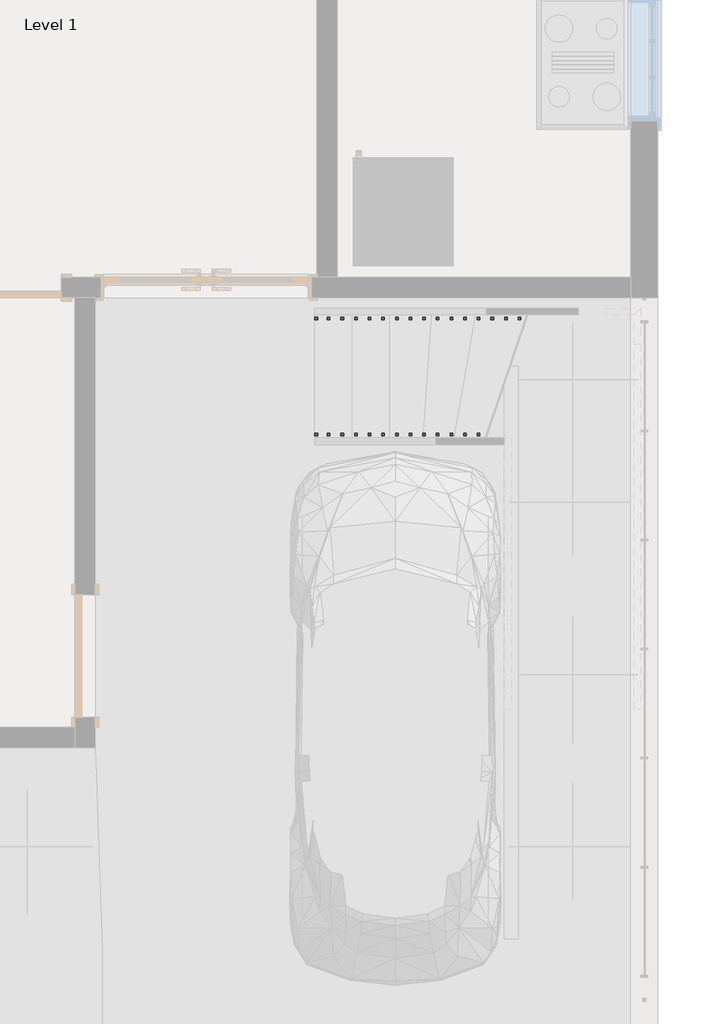
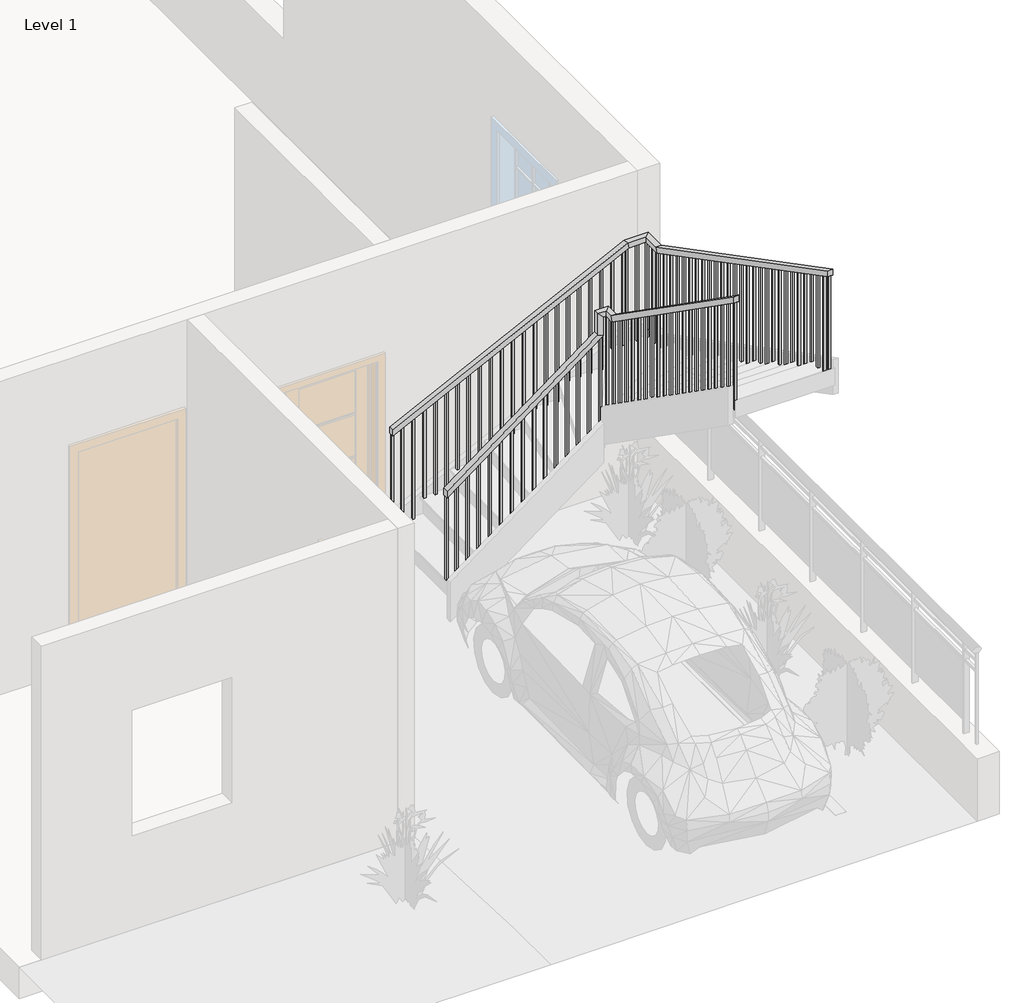
# One storey, part 2 of 3: 2 railings.
"""IFC4 building model written with IfcOpenShell, lengths in millimetres."""

from ifc_helpers import new_model, si_unit, frame, origin, place, context, project, spatial, polyline, outline, extrude, faceted_brep, element, save

model = new_model("IFC4")

# Units and contexts
model_context = context("Model", 3, world=origin())
ifc_project = project(units=[si_unit("LENGTHUNIT", "METRE", prefix="MILLI")], contexts=[model_context])

# Site, building, storey
site = spatial("IfcSite", under=ifc_project)
building = spatial("IfcBuilding", under=site)
storey = spatial("IfcBuildingStorey", under=building, Name="Level 1", Elevation=0.0)

# Railings
placement = place(None, origin())
element("IfcRailing", 1, ObjectType="Handrail - Rectangular", at=placement, inside=storey, context=model_context, shape_type="SolidModel", body=[
    faceted_brep([(2176.6969821, -750.949605, 1382.8377299), (2176.6969821, -750.949605, 1319.4090472), (2176.6969821, -801.749605, 1319.4090472), (2176.6969821, -801.749605, 1382.8377299), (3563.2339716, -750.949605, 2419.4929952), (3614.0339716, -750.949605, 2394.0453313), (3614.0339716, -801.749605, 2394.0453313), (3563.2339716, -801.749605, 2419.4929952), (3563.2339716, -750.949605, 2625.457216), (3614.0339716, -750.949605, 2574.657216), (3614.0339716, -801.749605, 2574.657216), (3563.2339716, -801.749605, 2625.457216), (3690.2339716, -750.949605, 2625.457216), (3690.2339716, -750.949605, 2574.657216), (3639.4339716, -801.749605, 2574.657216), (3639.4339716, -801.749605, 2625.457216), (3690.2339716, -877.949605, 2625.457216), (3690.2339716, -893.9792408, 2574.657216), (3639.4339716, -893.9792408, 2574.657216), (3639.4339716, -877.949605, 2625.457216), (3690.2339716, -2823.2865945, 3988.8904479), (3639.4339716, -2823.2865945, 3988.8904479), (3639.4339716, -2823.2865945, 3926.8557166), (3690.2339716, -2823.2865945, 3926.8557166)], [[[0, 1, 2, 3]], [[1, 0, 4, 5]], [[2, 1, 5, 6]], [[3, 2, 6, 7]], [[0, 3, 7, 4]], [[5, 4, 8, 9]], [[6, 5, 9, 10]], [[7, 6, 10, 11]], [[4, 7, 11, 8]], [[9, 8, 12, 13]], [[10, 9, 13, 14]], [[11, 10, 14, 15]], [[8, 11, 15, 12]], [[13, 12, 16, 17]], [[14, 13, 17, 18]], [[15, 14, 18, 19]], [[12, 15, 19, 16]], [[20, 21, 22, 23]], [[17, 16, 20, 23]], [[18, 17, 23, 22]], [[19, 18, 22, 21]], [[16, 19, 21, 20]]]),
    extrude(outline(polyline([(-2817.874605, 3923.0626019), (-2798.824605, 3909.7109805), (-2798.824605, 2878.6666667), (-2817.874605, 2878.6666667), (-2817.874605, 3923.0626019)])), frame((3655.3089716, 0.0, 0.0), z_axis=(1.0, 0.0, 0.0), x_axis=(0.0, 1.0, 0.0)), (0.0, 0.0, 1.0), 19.05),
    extrude(outline(polyline([(-2716.274605, 3851.8539542), (-2697.224605, 3838.5023328), (-2697.224605, 2878.6666667), (-2716.274605, 2878.6666667), (-2716.274605, 3851.8539542)])), frame((3655.3089716, 0.0, 0.0), z_axis=(1.0, 0.0, 0.0), x_axis=(0.0, 1.0, 0.0)), (0.0, 0.0, 1.0), 19.05),
    extrude(outline(polyline([(-2614.674605, 3780.7235858), (-2595.624605, 3767.3719643), (-2595.624605, 2878.6666667), (-2614.674605, 2878.6666667), (-2614.674605, 3780.7235858)])), frame((3655.3089716, 0.0, 0.0), z_axis=(1.0, 0.0, 0.0), x_axis=(0.0, 1.0, 0.0)), (0.0, 0.0, 1.0), 19.05),
    extrude(outline(polyline([(-2513.074605, 3709.514938), (-2494.024605, 3696.1633166), (-2494.024605, 2709.3333333), (-2513.074605, 2709.3333333), (-2513.074605, 3709.514938)])), frame((3655.3089716, 0.0, 0.0), z_axis=(1.0, 0.0, 0.0), x_axis=(0.0, 1.0, 0.0)), (0.0, 0.0, 1.0), 19.05),
    extrude(outline(polyline([(-2411.474605, 3638.3062903), (-2392.424605, 3624.9546689), (-2392.424605, 2709.3333333), (-2411.474605, 2709.3333333), (-2411.474605, 3638.3062903)])), frame((3655.3089716, 0.0, 0.0), z_axis=(1.0, 0.0, 0.0), x_axis=(0.0, 1.0, 0.0)), (0.0, 0.0, 1.0), 19.05),
    extrude(outline(polyline([(-2309.874605, 3567.0193634), (-2290.824605, 3553.667742), (-2290.824605, 2709.3333333), (-2309.874605, 2709.3333333), (-2309.874605, 3567.0193634)])), frame((3655.3089716, 0.0, 0.0), z_axis=(1.0, 0.0, 0.0), x_axis=(0.0, 1.0, 0.0)), (0.0, 0.0, 1.0), 19.05),
    extrude(outline(polyline([(-2208.274605, 3495.8889949), (-2189.224605, 3482.5373735), (-2189.224605, 2540.0), (-2208.274605, 2540.0), (-2208.274605, 3495.8889949)])), frame((3655.3089716, 0.0, 0.0), z_axis=(1.0, 0.0, 0.0), x_axis=(0.0, 1.0, 0.0)), (0.0, 0.0, 1.0), 19.05),
    extrude(outline(polyline([(-2106.674605, 3424.602068), (-2087.624605, 3411.2504466), (-2087.624605, 2540.0), (-2106.674605, 2540.0), (-2106.674605, 3424.602068)])), frame((3655.3089716, 0.0, 0.0), z_axis=(1.0, 0.0, 0.0), x_axis=(0.0, 1.0, 0.0)), (0.0, 0.0, 1.0), 19.05),
    extrude(outline(polyline([(-2005.074605, 3353.4716995), (-1986.024605, 3340.1200781), (-1986.024605, 2370.6666667), (-2005.074605, 2370.6666667), (-2005.074605, 3353.4716995)])), frame((3655.3089716, 0.0, 0.0), z_axis=(1.0, 0.0, 0.0), x_axis=(0.0, 1.0, 0.0)), (0.0, 0.0, 1.0), 19.05),
    extrude(outline(polyline([(-1903.474605, 3282.1847726), (-1884.424605, 3268.8331511), (-1884.424605, 2370.6666667), (-1903.474605, 2370.6666667), (-1903.474605, 3282.1847726)])), frame((3655.3089716, 0.0, 0.0), z_axis=(1.0, 0.0, 0.0), x_axis=(0.0, 1.0, 0.0)), (0.0, 0.0, 1.0), 19.05),
    extrude(outline(polyline([(-1801.874605, 3210.9761249), (-1782.824605, 3197.6245034), (-1782.824605, 2370.6666667), (-1801.874605, 2370.6666667), (-1801.874605, 3210.9761249)])), frame((3655.3089716, 0.0, 0.0), z_axis=(1.0, 0.0, 0.0), x_axis=(0.0, 1.0, 0.0)), (0.0, 0.0, 1.0), 19.05),
    extrude(outline(polyline([(-1700.274605, 3139.8457564), (-1681.224605, 3126.494135), (-1681.224605, 2201.3333333), (-1700.274605, 2201.3333333), (-1700.274605, 3139.8457564)])), frame((3655.3089716, 0.0, 0.0), z_axis=(1.0, 0.0, 0.0), x_axis=(0.0, 1.0, 0.0)), (0.0, 0.0, 1.0), 19.05),
    extrude(outline(polyline([(-1598.674605, 3068.5588295), (-1579.624605, 3055.207208), (-1579.624605, 2201.3333333), (-1598.674605, 2201.3333333), (-1598.674605, 3068.5588295)])), frame((3655.3089716, 0.0, 0.0), z_axis=(1.0, 0.0, 0.0), x_axis=(0.0, 1.0, 0.0)), (0.0, 0.0, 1.0), 19.05),
    extrude(outline(polyline([(-1497.074605, 2997.3501818), (-1478.024605, 2983.9985603), (-1478.024605, 2201.3333333), (-1497.074605, 2201.3333333), (-1497.074605, 2997.3501818)])), frame((3655.3089716, 0.0, 0.0), z_axis=(1.0, 0.0, 0.0), x_axis=(0.0, 1.0, 0.0)), (0.0, 0.0, 1.0), 19.05),
    extrude(outline(polyline([(-1395.474605, 2926.1415341), (-1376.424605, 2912.7899126), (-1376.424605, 2032.0), (-1395.474605, 2032.0), (-1395.474605, 2926.1415341)])), frame((3655.3089716, 0.0, 0.0), z_axis=(1.0, 0.0, 0.0), x_axis=(0.0, 1.0, 0.0)), (0.0, 0.0, 1.0), 19.05),
    extrude(outline(polyline([(-1293.874605, 2854.9328864), (-1274.824605, 2841.5812649), (-1274.824605, 2032.0), (-1293.874605, 2032.0), (-1293.874605, 2854.9328864)])), frame((3655.3089716, 0.0, 0.0), z_axis=(1.0, 0.0, 0.0), x_axis=(0.0, 1.0, 0.0)), (0.0, 0.0, 1.0), 19.05),
    extrude(outline(polyline([(-1192.274605, 2783.8025179), (-1173.224605, 2770.4508964), (-1173.224605, 1862.6666667), (-1192.274605, 1862.6666667), (-1192.274605, 2783.8025179)])), frame((3655.3089716, 0.0, 0.0), z_axis=(1.0, 0.0, 0.0), x_axis=(0.0, 1.0, 0.0)), (0.0, 0.0, 1.0), 19.05),
    extrude(outline(polyline([(-1090.674605, 2712.515591), (-1071.624605, 2699.1639695), (-1071.624605, 1862.6666667), (-1090.674605, 1862.6666667), (-1090.674605, 2712.515591)])), frame((3655.3089716, 0.0, 0.0), z_axis=(1.0, 0.0, 0.0), x_axis=(0.0, 1.0, 0.0)), (0.0, 0.0, 1.0), 19.05),
    extrude(outline(polyline([(-989.074605, 2641.3852225), (-970.024605, 2628.033601), (-970.024605, 1693.3333333), (-989.074605, 1693.3333333), (-989.074605, 2641.3852225)])), frame((3655.3089716, 0.0, 0.0), z_axis=(1.0, 0.0, 0.0), x_axis=(0.0, 1.0, 0.0)), (0.0, 0.0, 1.0), 19.05),
    extrude(outline(polyline([(3655.3089716, -868.424605), (3674.3589716, -868.424605), (3674.3589716, -887.474605), (3655.3089716, -887.474605), (3655.3089716, -868.424605)])), frame((0.0, 0.0, 1693.3333333), z_axis=(0.0, 0.0, 1.0), x_axis=(1.0, 0.0, 0.0)), (0.0, 0.0, 1.0), 881.3238827),
    extrude(outline(polyline([(2389.9990149, 3608.6219821), (2375.7561328, 3589.5719821), (1354.6666667, 3589.5719821), (1354.6666667, 3608.6219821), (2389.9990149, 3608.6219821)])), frame((0.0, -785.874605, 0.0), z_axis=(0.0, 1.0, 0.0), x_axis=(0.0, 0.0, 1.0)), (0.0, 0.0, 1.0), 19.05),
    extrude(outline(polyline([(2314.0369772, 3507.0219821), (2299.7940952, 3487.9719821), (1354.6666667, 3487.9719821), (1354.6666667, 3507.0219821), (2314.0369772, 3507.0219821)])), frame((0.0, -785.874605, 0.0), z_axis=(0.0, 1.0, 0.0), x_axis=(0.0, 0.0, 1.0)), (0.0, 0.0, 1.0), 19.05),
    extrude(outline(polyline([(2238.0749396, 3405.4219821), (2223.8320576, 3386.3719821), (1185.3333333, 3386.3719821), (1185.3333333, 3405.4219821), (2238.0749396, 3405.4219821)])), frame((0.0, -785.874605, 0.0), z_axis=(0.0, 1.0, 0.0), x_axis=(0.0, 0.0, 1.0)), (0.0, 0.0, 1.0), 19.05),
    extrude(outline(polyline([(2162.112902, 3303.8219821), (2147.8700199, 3284.7719821), (1185.3333333, 3284.7719821), (1185.3333333, 3303.8219821), (2162.112902, 3303.8219821)])), frame((0.0, -785.874605, 0.0), z_axis=(0.0, 1.0, 0.0), x_axis=(0.0, 0.0, 1.0)), (0.0, 0.0, 1.0), 19.05),
    extrude(outline(polyline([(2086.1508644, 3202.2219821), (2071.9079823, 3183.1719821), (1016.0, 3183.1719821), (1016.0, 3202.2219821), (2086.1508644, 3202.2219821)])), frame((0.0, -785.874605, 0.0), z_axis=(0.0, 1.0, 0.0), x_axis=(0.0, 0.0, 1.0)), (0.0, 0.0, 1.0), 19.05),
    extrude(outline(polyline([(2010.1888268, 3100.6219821), (1995.9459447, 3081.5719821), (1016.0, 3081.5719821), (1016.0, 3100.6219821), (2010.1888268, 3100.6219821)])), frame((0.0, -785.874605, 0.0), z_axis=(0.0, 1.0, 0.0), x_axis=(0.0, 0.0, 1.0)), (0.0, 0.0, 1.0), 19.05),
    extrude(outline(polyline([(1934.2267891, 2999.0219821), (1919.9839071, 2979.9719821), (1016.0, 2979.9719821), (1016.0, 2999.0219821), (1934.2267891, 2999.0219821)])), frame((0.0, -785.874605, 0.0), z_axis=(0.0, 1.0, 0.0), x_axis=(0.0, 0.0, 1.0)), (0.0, 0.0, 1.0), 19.05),
    extrude(outline(polyline([(1858.2647515, 2897.4219821), (1844.0218695, 2878.3719821), (846.6666667, 2878.3719821), (846.6666667, 2897.4219821), (1858.2647515, 2897.4219821)])), frame((0.0, -785.874605, 0.0), z_axis=(0.0, 1.0, 0.0), x_axis=(0.0, 0.0, 1.0)), (0.0, 0.0, 1.0), 19.05),
    extrude(outline(polyline([(1782.3027139, 2795.8219821), (1768.0598319, 2776.7719821), (846.6666667, 2776.7719821), (846.6666667, 2795.8219821), (1782.3027139, 2795.8219821)])), frame((0.0, -785.874605, 0.0), z_axis=(0.0, 1.0, 0.0), x_axis=(0.0, 0.0, 1.0)), (0.0, 0.0, 1.0), 19.05),
    extrude(outline(polyline([(1706.3406763, 2694.2219821), (1692.0977942, 2675.1719821), (677.3333333, 2675.1719821), (677.3333333, 2694.2219821), (1706.3406763, 2694.2219821)])), frame((0.0, -785.874605, 0.0), z_axis=(0.0, 1.0, 0.0), x_axis=(0.0, 0.0, 1.0)), (0.0, 0.0, 1.0), 19.05),
    extrude(outline(polyline([(1630.3786387, 2592.6219821), (1616.1357566, 2573.5719821), (677.3333333, 2573.5719821), (677.3333333, 2592.6219821), (1630.3786387, 2592.6219821)])), frame((0.0, -785.874605, 0.0), z_axis=(0.0, 1.0, 0.0), x_axis=(0.0, 0.0, 1.0)), (0.0, 0.0, 1.0), 19.05),
    extrude(outline(polyline([(1554.4166011, 2491.0219821), (1540.173719, 2471.9719821), (677.3333333, 2471.9719821), (677.3333333, 2491.0219821), (1554.4166011, 2491.0219821)])), frame((0.0, -785.874605, 0.0), z_axis=(0.0, 1.0, 0.0), x_axis=(0.0, 0.0, 1.0)), (0.0, 0.0, 1.0), 19.05),
    extrude(outline(polyline([(1478.4545634, 2389.4219821), (1464.2116814, 2370.3719821), (508.0, 2370.3719821), (508.0, 2389.4219821), (1478.4545634, 2389.4219821)])), frame((0.0, -785.874605, 0.0), z_axis=(0.0, 1.0, 0.0), x_axis=(0.0, 0.0, 1.0)), (0.0, 0.0, 1.0), 19.05),
    extrude(outline(polyline([(1402.4925258, 2287.8219821), (1388.2496438, 2268.7719821), (508.0, 2268.7719821), (508.0, 2287.8219821), (1402.4925258, 2287.8219821)])), frame((0.0, -785.874605, 0.0), z_axis=(0.0, 1.0, 0.0), x_axis=(0.0, 0.0, 1.0)), (0.0, 0.0, 1.0), 19.05),
    extrude(outline(polyline([(3655.3089716, -766.824605), (3674.3589716, -766.824605), (3674.3589716, -785.874605), (3655.3089716, -785.874605), (3655.3089716, -766.824605)])), frame((0.0, 0.0, 1524.0), z_axis=(0.0, 0.0, 1.0), x_axis=(1.0, 0.0, 0.0)), (0.0, 0.0, 1.0), 1050.657216),
    extrude(outline(polyline([(-2823.2865945, 3926.8557166), (-2804.2365945, 3913.5040952), (-2804.2365945, 2878.6666667), (-2823.2865945, 2878.6666667), (-2823.2865945, 3926.8557166)])), frame((3655.3089716, 0.0, 0.0), z_axis=(1.0, 0.0, 0.0), x_axis=(0.0, 1.0, 0.0)), (0.0, 0.0, 1.0), 19.05),
    extrude(outline(polyline([(1333.6519292, 2195.7469821), (1319.4090472, 2176.6969821), (508.0, 2176.6969821), (508.0, 2195.7469821), (1333.6519292, 2195.7469821)])), frame((0.0, -785.874605, 0.0), z_axis=(0.0, 1.0, 0.0), x_axis=(0.0, 0.0, 1.0)), (0.0, 0.0, 1.0), 19.05),
])
element("IfcRailing", 2, ObjectType="Handrail - Rectangular", at=placement, inside=storey, context=model_context, shape_type="SolidModel", body=[
    faceted_brep([(2176.6969821, 112.650395, 1453.9609055), (2176.6969821, 112.650395, 1397.3206453), (2176.6969821, 61.850395, 1397.3206453), (2176.6969821, 61.850395, 1453.9609055), (4334.8314449, 112.650395, 2518.1392326), (4346.6753872, 112.650395, 2467.3392326), (4346.6753872, 61.850395, 2467.3392326), (4334.8314449, 61.850395, 2518.1392326), (4553.8339716, 112.650395, 2518.1392326), (4553.8339716, 112.650395, 2467.3392326), (4503.0339716, 61.850395, 2467.3392326), (4503.0339716, 61.850395, 2518.1392326), (4553.8339716, -96.042338, 2518.1392326), (4553.8339716, -108.4787326, 2467.3392326), (4503.0339716, -108.4787326, 2467.3392326), (4503.0339716, -96.042338, 2518.1392326), (4553.8339716, -2823.2865945, 3938.588476), (4503.0339716, -2823.2865945, 3938.588476), (4503.0339716, -2823.2865945, 3881.3111437), (4553.8339716, -2823.2865945, 3881.3111437)], [[[0, 1, 2, 3]], [[1, 0, 4, 5]], [[2, 1, 5, 6]], [[3, 2, 6, 7]], [[0, 3, 7, 4]], [[5, 4, 8, 9]], [[6, 5, 9, 10]], [[7, 6, 10, 11]], [[4, 7, 11, 8]], [[9, 8, 12, 13]], [[10, 9, 13, 14]], [[11, 10, 14, 15]], [[8, 11, 15, 12]], [[16, 17, 18, 19]], [[13, 12, 16, 19]], [[14, 13, 19, 18]], [[15, 14, 18, 17]], [[12, 15, 17, 16]]]),
    extrude(outline(polyline([(-2728.117338, 3831.7378118), (-2728.117338, 2878.6666667), (-2747.167338, 2878.6666667), (-2747.167338, 3841.6597534), (-2728.117338, 3831.7378118)])), frame((4518.9089716, 0.0, 0.0), z_axis=(1.0, 0.0, 0.0), x_axis=(0.0, 1.0, 0.0)), (0.0, 0.0, 1.0), 19.05),
    extrude(outline(polyline([(-2626.517338, 3778.8264686), (-2626.517338, 2878.6666667), (-2645.567338, 2878.6666667), (-2645.567338, 3788.7484102), (-2626.517338, 3778.8264686)])), frame((4518.9089716, 0.0, 0.0), z_axis=(1.0, 0.0, 0.0), x_axis=(0.0, 1.0, 0.0)), (0.0, 0.0, 1.0), 19.05),
    extrude(outline(polyline([(-2524.917338, 3725.9037687), (-2524.917338, 2709.3333333), (-2543.967338, 2709.3333333), (-2543.967338, 3735.8257102), (-2524.917338, 3725.9037687)])), frame((4518.9089716, 0.0, 0.0), z_axis=(1.0, 0.0, 0.0), x_axis=(0.0, 1.0, 0.0)), (0.0, 0.0, 1.0), 19.05),
    extrude(outline(polyline([(-2423.317338, 3672.9867471), (-2423.317338, 2709.3333333), (-2442.367338, 2709.3333333), (-2442.367338, 3682.9086887), (-2423.317338, 3672.9867471)])), frame((4518.9089716, 0.0, 0.0), z_axis=(1.0, 0.0, 0.0), x_axis=(0.0, 1.0, 0.0)), (0.0, 0.0, 1.0), 19.05),
    extrude(outline(polyline([(-2321.717338, 3620.0754039), (-2321.717338, 2709.3333333), (-2340.767338, 2709.3333333), (-2340.767338, 3629.9973455), (-2321.717338, 3620.0754039)])), frame((4518.9089716, 0.0, 0.0), z_axis=(1.0, 0.0, 0.0), x_axis=(0.0, 1.0, 0.0)), (0.0, 0.0, 1.0), 19.05),
    extrude(outline(polyline([(-2220.117338, 3567.152704), (-2220.117338, 2540.0), (-2239.167338, 2540.0), (-2239.167338, 3577.0746455), (-2220.117338, 3567.152704)])), frame((4518.9089716, 0.0, 0.0), z_axis=(1.0, 0.0, 0.0), x_axis=(0.0, 1.0, 0.0)), (0.0, 0.0, 1.0), 19.05),
    extrude(outline(polyline([(-2118.517338, 3514.2356824), (-2118.517338, 2540.0), (-2137.567338, 2540.0), (-2137.567338, 3524.157624), (-2118.517338, 3514.2356824)])), frame((4518.9089716, 0.0, 0.0), z_axis=(1.0, 0.0, 0.0), x_axis=(0.0, 1.0, 0.0)), (0.0, 0.0, 1.0), 19.05),
    extrude(outline(polyline([(-2016.917338, 3461.3186609), (-2016.917338, 2540.0), (-2035.967338, 2540.0), (-2035.967338, 3471.2406024), (-2016.917338, 3461.3186609)])), frame((4518.9089716, 0.0, 0.0), z_axis=(1.0, 0.0, 0.0), x_axis=(0.0, 1.0, 0.0)), (0.0, 0.0, 1.0), 19.05),
    extrude(outline(polyline([(-1915.317338, 3408.4073177), (-1915.317338, 2370.6666667), (-1934.367338, 2370.6666667), (-1934.367338, 3418.3292592), (-1915.317338, 3408.4073177)])), frame((4518.9089716, 0.0, 0.0), z_axis=(1.0, 0.0, 0.0), x_axis=(0.0, 1.0, 0.0)), (0.0, 0.0, 1.0), 19.05),
    extrude(outline(polyline([(-1813.717338, 3355.4846177), (-1813.717338, 2370.6666667), (-1832.767338, 2370.6666667), (-1832.767338, 3365.4065593), (-1813.717338, 3355.4846177)])), frame((4518.9089716, 0.0, 0.0), z_axis=(1.0, 0.0, 0.0), x_axis=(0.0, 1.0, 0.0)), (0.0, 0.0, 1.0), 19.05),
    extrude(outline(polyline([(-1712.117338, 3302.5732745), (-1712.117338, 2370.6666667), (-1731.167338, 2370.6666667), (-1731.167338, 3312.4952161), (-1712.117338, 3302.5732745)])), frame((4518.9089716, 0.0, 0.0), z_axis=(1.0, 0.0, 0.0), x_axis=(0.0, 1.0, 0.0)), (0.0, 0.0, 1.0), 19.05),
    extrude(outline(polyline([(-1610.517338, 3249.656253), (-1610.517338, 2201.3333333), (-1629.567338, 2201.3333333), (-1629.567338, 3259.5781945), (-1610.517338, 3249.656253)])), frame((4518.9089716, 0.0, 0.0), z_axis=(1.0, 0.0, 0.0), x_axis=(0.0, 1.0, 0.0)), (0.0, 0.0, 1.0), 19.05),
    extrude(outline(polyline([(-1508.917338, 3196.7392314), (-1508.917338, 2201.3333333), (-1527.967338, 2201.3333333), (-1527.967338, 3206.661173), (-1508.917338, 3196.7392314)])), frame((4518.9089716, 0.0, 0.0), z_axis=(1.0, 0.0, 0.0), x_axis=(0.0, 1.0, 0.0)), (0.0, 0.0, 1.0), 19.05),
    extrude(outline(polyline([(-1407.317338, 3143.8222099), (-1407.317338, 2201.3333333), (-1426.367338, 2201.3333333), (-1426.367338, 3153.7441514), (-1407.317338, 3143.8222099)])), frame((4518.9089716, 0.0, 0.0), z_axis=(1.0, 0.0, 0.0), x_axis=(0.0, 1.0, 0.0)), (0.0, 0.0, 1.0), 19.05),
    extrude(outline(polyline([(-1305.717338, 3090.9051883), (-1305.717338, 2032.0), (-1324.767338, 2032.0), (-1324.767338, 3100.8271298), (-1305.717338, 3090.9051883)])), frame((4518.9089716, 0.0, 0.0), z_axis=(1.0, 0.0, 0.0), x_axis=(0.0, 1.0, 0.0)), (0.0, 0.0, 1.0), 19.05),
    extrude(outline(polyline([(-1204.117338, 3037.9881667), (-1204.117338, 2032.0), (-1223.167338, 2032.0), (-1223.167338, 3047.9101083), (-1204.117338, 3037.9881667)])), frame((4518.9089716, 0.0, 0.0), z_axis=(1.0, 0.0, 0.0), x_axis=(0.0, 1.0, 0.0)), (0.0, 0.0, 1.0), 19.05),
    extrude(outline(polyline([(-1102.517338, 2985.0711452), (-1102.517338, 2032.0), (-1121.567338, 2032.0), (-1121.567338, 2994.9930867), (-1102.517338, 2985.0711452)])), frame((4518.9089716, 0.0, 0.0), z_axis=(1.0, 0.0, 0.0), x_axis=(0.0, 1.0, 0.0)), (0.0, 0.0, 1.0), 19.05),
    extrude(outline(polyline([(-1000.917338, 2932.1541236), (-1000.917338, 1862.6666667), (-1019.967338, 1862.6666667), (-1019.967338, 2942.0760651), (-1000.917338, 2932.1541236)])), frame((4518.9089716, 0.0, 0.0), z_axis=(1.0, 0.0, 0.0), x_axis=(0.0, 1.0, 0.0)), (0.0, 0.0, 1.0), 19.05),
    extrude(outline(polyline([(-899.317338, 2879.237102), (-899.317338, 1862.6666667), (-918.367338, 1862.6666667), (-918.367338, 2889.1590436), (-899.317338, 2879.237102)])), frame((4518.9089716, 0.0, 0.0), z_axis=(1.0, 0.0, 0.0), x_axis=(0.0, 1.0, 0.0)), (0.0, 0.0, 1.0), 19.05),
    extrude(outline(polyline([(-797.717338, 2826.3200805), (-797.717338, 1862.6666667), (-816.767338, 1862.6666667), (-816.767338, 2836.242022), (-797.717338, 2826.3200805)])), frame((4518.9089716, 0.0, 0.0), z_axis=(1.0, 0.0, 0.0), x_axis=(0.0, 1.0, 0.0)), (0.0, 0.0, 1.0), 19.05),
    extrude(outline(polyline([(-696.117338, 2773.4030589), (-696.117338, 1693.3333333), (-715.167338, 1693.3333333), (-715.167338, 2783.3250004), (-696.117338, 2773.4030589)])), frame((4518.9089716, 0.0, 0.0), z_axis=(1.0, 0.0, 0.0), x_axis=(0.0, 1.0, 0.0)), (0.0, 0.0, 1.0), 19.05),
    extrude(outline(polyline([(-594.517338, 2720.4860373), (-594.517338, 1693.3333333), (-613.567338, 1693.3333333), (-613.567338, 2730.4079789), (-594.517338, 2720.4860373)])), frame((4518.9089716, 0.0, 0.0), z_axis=(1.0, 0.0, 0.0), x_axis=(0.0, 1.0, 0.0)), (0.0, 0.0, 1.0), 19.05),
    extrude(outline(polyline([(-492.917338, 2667.5690158), (-492.917338, 1693.3333333), (-511.967338, 1693.3333333), (-511.967338, 2677.4909573), (-492.917338, 2667.5690158)])), frame((4518.9089716, 0.0, 0.0), z_axis=(1.0, 0.0, 0.0), x_axis=(0.0, 1.0, 0.0)), (0.0, 0.0, 1.0), 19.05),
    extrude(outline(polyline([(-391.317338, 2614.6519942), (-391.317338, 1693.3333333), (-410.367338, 1693.3333333), (-410.367338, 2624.5739357), (-391.317338, 2614.6519942)])), frame((4518.9089716, 0.0, 0.0), z_axis=(1.0, 0.0, 0.0), x_axis=(0.0, 1.0, 0.0)), (0.0, 0.0, 1.0), 19.05),
    extrude(outline(polyline([(-289.717338, 2561.7349726), (-289.717338, 1693.3333333), (-308.767338, 1693.3333333), (-308.767338, 2571.6569142), (-289.717338, 2561.7349726)])), frame((4518.9089716, 0.0, 0.0), z_axis=(1.0, 0.0, 0.0), x_axis=(0.0, 1.0, 0.0)), (0.0, 0.0, 1.0), 19.05),
    extrude(outline(polyline([(-188.117338, 2508.8179511), (-188.117338, 1524.0), (-207.167338, 1524.0), (-207.167338, 2518.7398926), (-188.117338, 2508.8179511)])), frame((4518.9089716, 0.0, 0.0), z_axis=(1.0, 0.0, 0.0), x_axis=(0.0, 1.0, 0.0)), (0.0, 0.0, 1.0), 19.05),
    extrude(outline(polyline([(4537.9589716, -4.824605), (4537.9589716, -23.874605), (4518.9089716, -23.874605), (4518.9089716, -4.824605), (4537.9589716, -4.824605)])), frame((0.0, 0.0, 1524.0), z_axis=(0.0, 0.0, 1.0), x_axis=(1.0, 0.0, 0.0)), (0.0, 0.0, 1.0), 943.3392326),
    extrude(outline(polyline([(4426.9064449, 96.775395), (4445.9564449, 96.775395), (4445.9564449, 77.725395), (4426.9064449, 77.725395), (4426.9064449, 96.775395)])), frame((0.0, 0.0, 1524.0), z_axis=(0.0, 0.0, 1.0), x_axis=(1.0, 0.0, 0.0)), (0.0, 0.0, 1.0), 943.3392326),
    extrude(outline(polyline([(2444.7042162, 4300.7719821), (1524.0, 4300.7719821), (1524.0, 4319.8219821), (2454.0977908, 4319.8219821), (2444.7042162, 4300.7719821)])), frame((0.0, 77.725395, 0.0), z_axis=(0.0, 1.0, 0.0), x_axis=(0.0, 0.0, 1.0)), (0.0, 0.0, 1.0), 19.05),
    extrude(outline(polyline([(2394.6051515, 4199.1719821), (1524.0, 4199.1719821), (1524.0, 4218.2219821), (2403.9987262, 4218.2219821), (2394.6051515, 4199.1719821)])), frame((0.0, 77.725395, 0.0), z_axis=(0.0, 1.0, 0.0), x_axis=(0.0, 0.0, 1.0)), (0.0, 0.0, 1.0), 19.05),
    extrude(outline(polyline([(2344.5060869, 4097.5719821), (1354.6666667, 4097.5719821), (1354.6666667, 4116.6219821), (2353.8996615, 4116.6219821), (2344.5060869, 4097.5719821)])), frame((0.0, 77.725395, 0.0), z_axis=(0.0, 1.0, 0.0), x_axis=(0.0, 0.0, 1.0)), (0.0, 0.0, 1.0), 19.05),
    extrude(outline(polyline([(2294.4070222, 3995.9719821), (1354.6666667, 3995.9719821), (1354.6666667, 4015.0219821), (2303.8005968, 4015.0219821), (2294.4070222, 3995.9719821)])), frame((0.0, 77.725395, 0.0), z_axis=(0.0, 1.0, 0.0), x_axis=(0.0, 0.0, 1.0)), (0.0, 0.0, 1.0), 19.05),
    extrude(outline(polyline([(2244.3079575, 3894.3719821), (1354.6666667, 3894.3719821), (1354.6666667, 3913.4219821), (2253.7015321, 3913.4219821), (2244.3079575, 3894.3719821)])), frame((0.0, 77.725395, 0.0), z_axis=(0.0, 1.0, 0.0), x_axis=(0.0, 0.0, 1.0)), (0.0, 0.0, 1.0), 19.05),
    extrude(outline(polyline([(2194.2088928, 3792.7719821), (1354.6666667, 3792.7719821), (1354.6666667, 3811.8219821), (2203.6024675, 3811.8219821), (2194.2088928, 3792.7719821)])), frame((0.0, 77.725395, 0.0), z_axis=(0.0, 1.0, 0.0), x_axis=(0.0, 0.0, 1.0)), (0.0, 0.0, 1.0), 19.05),
    extrude(outline(polyline([(2144.1098282, 3691.1719821), (1185.3333333, 3691.1719821), (1185.3333333, 3710.2219821), (2153.5034028, 3710.2219821), (2144.1098282, 3691.1719821)])), frame((0.0, 77.725395, 0.0), z_axis=(0.0, 1.0, 0.0), x_axis=(0.0, 0.0, 1.0)), (0.0, 0.0, 1.0), 19.05),
    extrude(outline(polyline([(2094.0107635, 3589.5719821), (1185.3333333, 3589.5719821), (1185.3333333, 3608.6219821), (2103.4043381, 3608.6219821), (2094.0107635, 3589.5719821)])), frame((0.0, 77.725395, 0.0), z_axis=(0.0, 1.0, 0.0), x_axis=(0.0, 0.0, 1.0)), (0.0, 0.0, 1.0), 19.05),
    extrude(outline(polyline([(2043.9116988, 3487.9719821), (1185.3333333, 3487.9719821), (1185.3333333, 3507.0219821), (2053.3052734, 3507.0219821), (2043.9116988, 3487.9719821)])), frame((0.0, 77.725395, 0.0), z_axis=(0.0, 1.0, 0.0), x_axis=(0.0, 0.0, 1.0)), (0.0, 0.0, 1.0), 19.05),
    extrude(outline(polyline([(1993.8126341, 3386.3719821), (1185.3333333, 3386.3719821), (1185.3333333, 3405.4219821), (2003.2062088, 3405.4219821), (1993.8126341, 3386.3719821)])), frame((0.0, 77.725395, 0.0), z_axis=(0.0, 1.0, 0.0), x_axis=(0.0, 0.0, 1.0)), (0.0, 0.0, 1.0), 19.05),
    extrude(outline(polyline([(1943.7135694, 3284.7719821), (1016.0, 3284.7719821), (1016.0, 3303.8219821), (1953.1071441, 3303.8219821), (1943.7135694, 3284.7719821)])), frame((0.0, 77.725395, 0.0), z_axis=(0.0, 1.0, 0.0), x_axis=(0.0, 0.0, 1.0)), (0.0, 0.0, 1.0), 19.05),
    extrude(outline(polyline([(1893.6145048, 3183.1719821), (1016.0, 3183.1719821), (1016.0, 3202.2219821), (1903.0080794, 3202.2219821), (1893.6145048, 3183.1719821)])), frame((0.0, 77.725395, 0.0), z_axis=(0.0, 1.0, 0.0), x_axis=(0.0, 0.0, 1.0)), (0.0, 0.0, 1.0), 19.05),
    extrude(outline(polyline([(1843.5154401, 3081.5719821), (1016.0, 3081.5719821), (1016.0, 3100.6219821), (1852.9090147, 3100.6219821), (1843.5154401, 3081.5719821)])), frame((0.0, 77.725395, 0.0), z_axis=(0.0, 1.0, 0.0), x_axis=(0.0, 0.0, 1.0)), (0.0, 0.0, 1.0), 19.05),
    extrude(outline(polyline([(1793.4163754, 2979.9719821), (846.6666667, 2979.9719821), (846.6666667, 2999.0219821), (1802.80995, 2999.0219821), (1793.4163754, 2979.9719821)])), frame((0.0, 77.725395, 0.0), z_axis=(0.0, 1.0, 0.0), x_axis=(0.0, 0.0, 1.0)), (0.0, 0.0, 1.0), 19.05),
    extrude(outline(polyline([(1743.3173107, 2878.3719821), (846.6666667, 2878.3719821), (846.6666667, 2897.4219821), (1752.7108854, 2897.4219821), (1743.3173107, 2878.3719821)])), frame((0.0, 77.725395, 0.0), z_axis=(0.0, 1.0, 0.0), x_axis=(0.0, 0.0, 1.0)), (0.0, 0.0, 1.0), 19.05),
    extrude(outline(polyline([(1693.2182461, 2776.7719821), (846.6666667, 2776.7719821), (846.6666667, 2795.8219821), (1702.6118207, 2795.8219821), (1693.2182461, 2776.7719821)])), frame((0.0, 77.725395, 0.0), z_axis=(0.0, 1.0, 0.0), x_axis=(0.0, 0.0, 1.0)), (0.0, 0.0, 1.0), 19.05),
    extrude(outline(polyline([(1643.1191814, 2675.1719821), (677.3333333, 2675.1719821), (677.3333333, 2694.2219821), (1652.512756, 2694.2219821), (1643.1191814, 2675.1719821)])), frame((0.0, 77.725395, 0.0), z_axis=(0.0, 1.0, 0.0), x_axis=(0.0, 0.0, 1.0)), (0.0, 0.0, 1.0), 19.05),
    extrude(outline(polyline([(1593.0201167, 2573.5719821), (677.3333333, 2573.5719821), (677.3333333, 2592.6219821), (1602.4136913, 2592.6219821), (1593.0201167, 2573.5719821)])), frame((0.0, 77.725395, 0.0), z_axis=(0.0, 1.0, 0.0), x_axis=(0.0, 0.0, 1.0)), (0.0, 0.0, 1.0), 19.05),
    extrude(outline(polyline([(1542.921052, 2471.9719821), (677.3333333, 2471.9719821), (677.3333333, 2491.0219821), (1552.3146267, 2491.0219821), (1542.921052, 2471.9719821)])), frame((0.0, 77.725395, 0.0), z_axis=(0.0, 1.0, 0.0), x_axis=(0.0, 0.0, 1.0)), (0.0, 0.0, 1.0), 19.05),
    extrude(outline(polyline([(1492.8219874, 2370.3719821), (508.0, 2370.3719821), (508.0, 2389.4219821), (1502.215562, 2389.4219821), (1492.8219874, 2370.3719821)])), frame((0.0, 77.725395, 0.0), z_axis=(0.0, 1.0, 0.0), x_axis=(0.0, 0.0, 1.0)), (0.0, 0.0, 1.0), 19.05),
    extrude(outline(polyline([(1442.7229227, 2268.7719821), (508.0, 2268.7719821), (508.0, 2287.8219821), (1452.1164973, 2287.8219821), (1442.7229227, 2268.7719821)])), frame((0.0, 77.725395, 0.0), z_axis=(0.0, 1.0, 0.0), x_axis=(0.0, 0.0, 1.0)), (0.0, 0.0, 1.0), 19.05),
    extrude(outline(polyline([(4537.9589716, -86.517338), (4537.9589716, -105.567338), (4518.9089716, -105.567338), (4518.9089716, -86.517338), (4537.9589716, -86.517338)])), frame((0.0, 0.0, 1524.0), z_axis=(0.0, 0.0, 1.0), x_axis=(1.0, 0.0, 0.0)), (0.0, 0.0, 1.0), 943.3392326),
    extrude(outline(polyline([(4518.9089716, 96.775395), (4537.9589716, 96.775395), (4537.9589716, 77.725395), (4518.9089716, 77.725395), (4518.9089716, 96.775395)])), frame((0.0, 0.0, 1524.0), z_axis=(0.0, 0.0, 1.0), x_axis=(1.0, 0.0, 0.0)), (0.0, 0.0, 1.0), 943.3392326),
    extrude(outline(polyline([(2456.8021851, 4325.3064449), (1524.0, 4325.3064449), (1524.0, 4344.3564449), (2466.1957597, 4344.3564449), (2456.8021851, 4325.3064449)])), frame((0.0, 77.725395, 0.0), z_axis=(0.0, 1.0, 0.0), x_axis=(0.0, 0.0, 1.0)), (0.0, 0.0, 1.0), 19.05),
    extrude(outline(polyline([(-2804.2365945, 3871.3892021), (-2804.2365945, 2878.6666667), (-2823.2865945, 2878.6666667), (-2823.2865945, 3881.3111437), (-2804.2365945, 3871.3892021)])), frame((4518.9089716, 0.0, 0.0), z_axis=(1.0, 0.0, 0.0), x_axis=(0.0, 1.0, 0.0)), (0.0, 0.0, 1.0), 19.05),
    extrude(outline(polyline([(1397.3206453, 2176.6969821), (508.0, 2176.6969821), (508.0, 2195.7469821), (1406.7142199, 2195.7469821), (1397.3206453, 2176.6969821)])), frame((0.0, 77.725395, 0.0), z_axis=(0.0, 1.0, 0.0), x_axis=(0.0, 0.0, 1.0)), (0.0, 0.0, 1.0), 19.05),
])

save(model, "model.ifc")

# Revit data of these elements
# Type "Handrail - Rectangular"
#   Assembly Code = "C2010400"
#   built-in parameter 1008612 = 0.0416667 (stored number, unit not read)
#   built-in parameter 1008611 = 0.0416667 (stored number, unit not read)
#   built-in parameter 1008609 = 0.333333 (stored number, unit not read)
#   built-in parameter 1008604 = 0.166667 (stored number, unit not read)
#   built-in parameter 1008603 = 0.166667 (stored number, unit not read)
#   Railing Height = 3' - 0"
#   built-in parameter 1008630 = 2
#   built-in parameter 1008610 = 2
#   built-in parameter 1008618 = Baluster - Square : 3/4"
# Elements 1, 2 (IfcRailing, "Handrail - Rectangular")
#   Phase Created = New Construction
